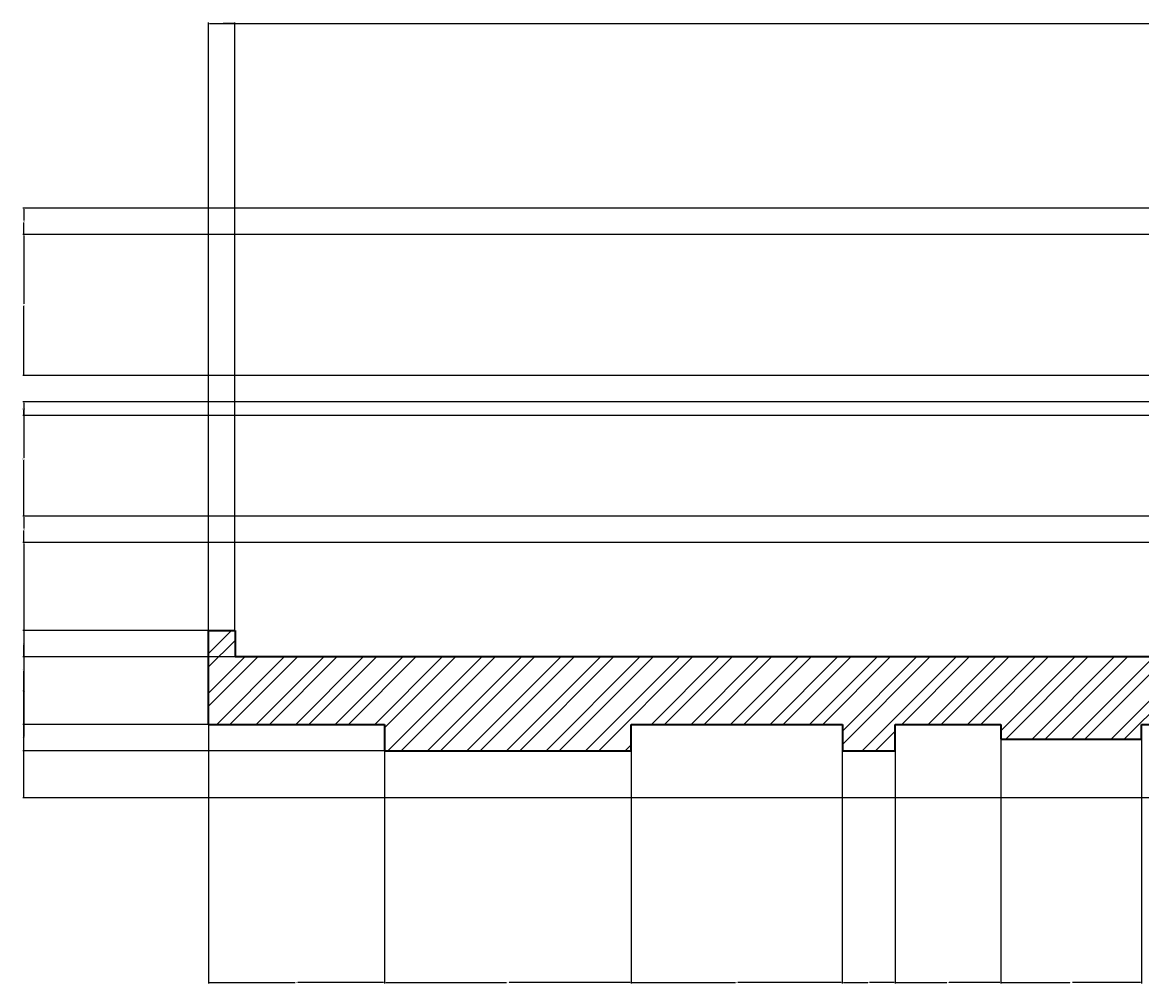
# Model space of a CAD drawing. Units: inches. Extents: x 2121 to 2815, y 1818 to 2233.
# Tile 3 of 6: x 2121 to 2312, y 2070 to 2233. Entities that reach past the tile are written whole.
import ezdxf

# ---------------------------------------------------------------- set-up
doc = ezdxf.new("R2010")
doc.units = ezdxf.units.IN
for name, color, linetype, lineweight in [('A-ANNO-DIMS', 2, 'Continuous', 18), ('A-WALL', 7, 'Continuous', 35), ('A-WALL-PATT', 8, 'Continuous', 13)]:
    doc.layers.add(name, color=color, linetype=linetype, lineweight=lineweight)
doc.styles.get("Standard").update_dxf_attribs({"font": 'arial.ttf'})
doc.dimstyles.get("Standard").update_dxf_attribs({"dimtxt": 0.18, "dimasz": 0.18, "dimexe": 0.18, "dimexo": 0.0625, "dimgap": 0.09, "dimtad": 0, "dimtih": 1, "dimtoh": 1, "dimdec": 4, "dimzin": 0, "dimdsep": 46, "dimtxsty": 'Standard', "dimcen": 0.09, "dimadec": 0, "dimazin": 0, "dimtfac": 1, "dimtdec": 4, "dimtofl": 0, "dimtmove": 0, "dimatfit": 3, "dimfxl": 1, "dimtolj": 1, "dimtzin": 0, "dimarcsym": 0})

# ---------------------------------------------------------------- blocks, each defined once
blk = doc.blocks.new('*D10')
at = {"layer": 'A-ANNO-DIMS', "color": 0, "lineweight": -2, "transparency": 16777216}
for p, q in [((2152.83, 2129.87), (2152.83, 2233.48)), ((2153.01, 2233.3), (2396.54, 2233.3)), ((2640.65, 2233.3), (2397.13, 2233.3)), ((2640.83, 2129.87), (2640.83, 2233.48))]:
    blk.add_line(p, q, dxfattribs=at)
at = {"layer": 'A-ANNO-DIMS', "color": 0, "transparency": 16777216}
for points in [[(2153.01, 2233.33), (2153.01, 2233.27), (2152.83, 2233.3)], [(2640.65, 2233.33), (2640.65, 2233.27), (2640.83, 2233.3)]]:
    blk.add_solid(points, dxfattribs=at)
at = {"layer": 'Defpoints', "color": 0, "transparency": 16777216}
for p in [(2640.83, 2233.3), (2152.83, 2129.81), (2640.83, 2129.81)]:
    blk.add_point(p, dxfattribs=at)
at = {"layer": 'A-ANNO-DIMS', "color": 0, "transparency": 16777216, "insert": (2396.83, 2233.3), "char_height": 0.18, "attachment_point": 5}
blk.add_mtext('\\A1;488', dxfattribs=at)
blk = doc.blocks.new('*D12')
at = {"layer": 'A-ANNO-DIMS', "color": 0, "lineweight": -2, "transparency": 16777216}
for p, q in [((2152.83, 2113.75), (2152.83, 2069.63)), ((2182.83, 2109.25), (2182.83, 2069.63)), ((2153.01, 2069.81), (2167.61, 2069.81)), ((2182.65, 2069.81), (2168.05, 2069.81))]:
    blk.add_line(p, q, dxfattribs=at)
at = {"layer": 'A-ANNO-DIMS', "color": 0, "transparency": 16777216}
for points in [[(2153.01, 2069.84), (2153.01, 2069.78), (2152.83, 2069.81)], [(2182.65, 2069.84), (2182.65, 2069.78), (2182.83, 2069.81)]]:
    blk.add_solid(points, dxfattribs=at)
at = {"layer": 'Defpoints', "color": 0, "transparency": 16777216}
for p in [(2152.83, 2113.81), (2182.83, 2109.31), (2182.83, 2069.81)]:
    blk.add_point(p, dxfattribs=at)
at = {"layer": 'A-ANNO-DIMS', "color": 0, "transparency": 16777216, "insert": (2167.83, 2069.81), "char_height": 0.18, "attachment_point": 5}
blk.add_mtext('\\A1;30', dxfattribs=at)
blk = doc.blocks.new('*D13')
at = {"layer": 'A-ANNO-DIMS', "color": 0, "lineweight": -2, "transparency": 16777216}
for p, q in [((2182.83, 2109.25), (2182.83, 2069.63)), ((2224.83, 2109.25), (2224.83, 2069.63)), ((2183.01, 2069.81), (2203.61, 2069.81)), ((2224.65, 2069.81), (2204.05, 2069.81))]:
    blk.add_line(p, q, dxfattribs=at)
at = {"layer": 'A-ANNO-DIMS', "color": 0, "transparency": 16777216}
for points in [[(2183.01, 2069.84), (2183.01, 2069.78), (2182.83, 2069.81)], [(2224.65, 2069.84), (2224.65, 2069.78), (2224.83, 2069.81)]]:
    blk.add_solid(points, dxfattribs=at)
at = {"layer": 'Defpoints', "color": 0, "transparency": 16777216}
for p in [(2182.83, 2109.31), (2224.83, 2109.31), (2224.83, 2069.81)]:
    blk.add_point(p, dxfattribs=at)
at = {"layer": 'A-ANNO-DIMS', "color": 0, "transparency": 16777216, "insert": (2203.83, 2069.81), "char_height": 0.18, "attachment_point": 5}
blk.add_mtext('\\A1;42', dxfattribs=at)
blk = doc.blocks.new('*D14')
at = {"layer": 'A-ANNO-DIMS', "color": 0, "lineweight": -2, "transparency": 16777216}
for p, q in [((2224.83, 2109.25), (2224.83, 2069.63)), ((2260.83, 2109.25), (2260.83, 2069.63)), ((2225.01, 2069.81), (2242.61, 2069.81)), ((2260.65, 2069.81), (2243.05, 2069.81))]:
    blk.add_line(p, q, dxfattribs=at)
at = {"layer": 'A-ANNO-DIMS', "color": 0, "transparency": 16777216}
for points in [[(2225.01, 2069.84), (2225.01, 2069.78), (2224.83, 2069.81)], [(2260.65, 2069.84), (2260.65, 2069.78), (2260.83, 2069.81)]]:
    blk.add_solid(points, dxfattribs=at)
at = {"layer": 'Defpoints', "color": 0, "transparency": 16777216}
for p in [(2224.83, 2109.31), (2260.83, 2109.31), (2260.83, 2069.81)]:
    blk.add_point(p, dxfattribs=at)
at = {"layer": 'A-ANNO-DIMS', "color": 0, "transparency": 16777216, "insert": (2242.83, 2069.81), "char_height": 0.18, "attachment_point": 5}
blk.add_mtext('\\A1;36', dxfattribs=at)
blk = doc.blocks.new('*D15')
at = {"layer": 'A-ANNO-DIMS', "color": 0, "lineweight": -2, "transparency": 16777216}
for p, q in [((2260.83, 2109.25), (2260.83, 2069.63)), ((2269.83, 2109.25), (2269.83, 2069.63)), ((2261.01, 2069.81), (2265.18, 2069.81)), ((2269.65, 2069.81), (2265.48, 2069.81))]:
    blk.add_line(p, q, dxfattribs=at)
at = {"layer": 'A-ANNO-DIMS', "color": 0, "transparency": 16777216}
for points in [[(2261.01, 2069.84), (2261.01, 2069.78), (2260.83, 2069.81)], [(2269.65, 2069.84), (2269.65, 2069.78), (2269.83, 2069.81)]]:
    blk.add_solid(points, dxfattribs=at)
at = {"layer": 'Defpoints', "color": 0, "transparency": 16777216}
for p in [(2260.83, 2109.31), (2269.83, 2109.31), (2269.83, 2069.81)]:
    blk.add_point(p, dxfattribs=at)
at = {"layer": 'A-ANNO-DIMS', "color": 0, "transparency": 16777216, "insert": (2265.33, 2069.81), "char_height": 0.18, "attachment_point": 5}
blk.add_mtext('\\A1;9', dxfattribs=at)
blk = doc.blocks.new('*D16')
at = {"layer": 'A-ANNO-DIMS', "color": 0, "lineweight": -2, "transparency": 16777216}
for p, q in [((2287.83, 2111.25), (2287.83, 2069.63)), ((2269.83, 2109.25), (2269.83, 2069.63)), ((2270.01, 2069.81), (2278.62, 2069.81)), ((2287.65, 2069.81), (2279.04, 2069.81))]:
    blk.add_line(p, q, dxfattribs=at)
at = {"layer": 'A-ANNO-DIMS', "color": 0, "transparency": 16777216}
for points in [[(2270.01, 2069.84), (2270.01, 2069.78), (2269.83, 2069.81)], [(2287.65, 2069.84), (2287.65, 2069.78), (2287.83, 2069.81)]]:
    blk.add_solid(points, dxfattribs=at)
at = {"layer": 'Defpoints', "color": 0, "transparency": 16777216}
for p in [(2287.83, 2111.31), (2269.83, 2109.31), (2287.83, 2069.81)]:
    blk.add_point(p, dxfattribs=at)
at = {"layer": 'A-ANNO-DIMS', "color": 0, "transparency": 16777216, "insert": (2278.83, 2069.81), "char_height": 0.18, "attachment_point": 5}
blk.add_mtext('\\A1;18', dxfattribs=at)
blk = doc.blocks.new('*D17')
at = {"layer": 'A-ANNO-DIMS', "color": 0, "lineweight": -2, "transparency": 16777216}
for p, q in [((2287.83, 2111.25), (2287.83, 2069.63)), ((2311.83, 2111.25), (2311.83, 2069.63)), ((2288.01, 2069.81), (2299.61, 2069.81)), ((2311.65, 2069.81), (2300.05, 2069.81))]:
    blk.add_line(p, q, dxfattribs=at)
at = {"layer": 'A-ANNO-DIMS', "color": 0, "transparency": 16777216}
for points in [[(2288.01, 2069.84), (2288.01, 2069.78), (2287.83, 2069.81)], [(2311.65, 2069.84), (2311.65, 2069.78), (2311.83, 2069.81)]]:
    blk.add_solid(points, dxfattribs=at)
at = {"layer": 'Defpoints', "color": 0, "transparency": 16777216}
for p in [(2287.83, 2111.31), (2311.83, 2111.31), (2311.83, 2069.81)]:
    blk.add_point(p, dxfattribs=at)
at = {"layer": 'A-ANNO-DIMS', "color": 0, "transparency": 16777216, "insert": (2299.83, 2069.81), "char_height": 0.18, "attachment_point": 5}
blk.add_mtext('\\A1;24', dxfattribs=at)
blk = doc.blocks.new('*D28')
at = {"layer": 'A-ANNO-DIMS', "color": 0, "lineweight": -2, "transparency": 16777216}
for p, q in [((2152.83, 2129.87), (2152.83, 2233.48)), ((2153.01, 2233.3), (2154.82, 2233.3)), ((2157.15, 2233.3), (2155.34, 2233.3)), ((2157.33, 2129.87), (2157.33, 2233.48))]:
    blk.add_line(p, q, dxfattribs=at)
at = {"layer": 'A-ANNO-DIMS', "color": 0, "transparency": 16777216}
for points in [[(2153.01, 2233.33), (2153.01, 2233.27), (2152.83, 2233.3)], [(2157.15, 2233.33), (2157.15, 2233.27), (2157.33, 2233.3)]]:
    blk.add_solid(points, dxfattribs=at)
at = {"layer": 'Defpoints', "color": 0, "transparency": 16777216}
for p in [(2157.33, 2233.3), (2152.83, 2129.81), (2157.33, 2129.81)]:
    blk.add_point(p, dxfattribs=at)
at = {"layer": 'A-ANNO-DIMS', "color": 0, "transparency": 16777216, "insert": (2155.08, 2233.3), "char_height": 0.18, "attachment_point": 5}
blk.add_mtext('\\A1;4.5', dxfattribs=at)
blk = doc.blocks.new('*D29')
at = {"layer": 'A-ANNO-DIMS', "color": 0, "lineweight": -2, "transparency": 16777216}
for p, q in [((2157.27, 2129.81), (2121.16, 2129.81)), ((2121.34, 2129.63), (2121.34, 2127.74)), ((2121.34, 2125.49), (2121.34, 2127.38)), ((2157.27, 2125.31), (2121.16, 2125.31))]:
    blk.add_line(p, q, dxfattribs=at)
at = {"layer": 'A-ANNO-DIMS', "color": 0, "transparency": 16777216}
for points in [[(2121.31, 2129.63), (2121.37, 2129.63), (2121.34, 2129.81)], [(2121.31, 2125.49), (2121.37, 2125.49), (2121.34, 2125.31)]]:
    blk.add_solid(points, dxfattribs=at)
at = {"layer": 'Defpoints', "color": 0, "transparency": 16777216}
for p in [(2121.34, 2129.81), (2157.33, 2129.81), (2157.33, 2125.31)]:
    blk.add_point(p, dxfattribs=at)
at = {"layer": 'A-ANNO-DIMS', "color": 0, "transparency": 16777216, "insert": (2121.34, 2127.56), "char_height": 0.18, "attachment_point": 5}
blk.add_mtext('\\A1;4.5', dxfattribs=at)
blk = doc.blocks.new('*D30')
at = {"layer": 'A-ANNO-DIMS', "color": 0, "lineweight": -2, "transparency": 16777216}
for p, q in [((2157.27, 2125.31), (2121.16, 2125.31)), ((2121.34, 2125.13), (2121.34, 2119.74)), ((2121.34, 2113.99), (2121.34, 2119.38)), ((2152.77, 2113.81), (2121.16, 2113.81))]:
    blk.add_line(p, q, dxfattribs=at)
at = {"layer": 'A-ANNO-DIMS', "color": 0, "transparency": 16777216}
for points in [[(2121.31, 2125.13), (2121.37, 2125.13), (2121.34, 2125.31)], [(2121.31, 2113.99), (2121.37, 2113.99), (2121.34, 2113.81)]]:
    blk.add_solid(points, dxfattribs=at)
at = {"layer": 'Defpoints', "color": 0, "transparency": 16777216}
for p in [(2157.33, 2125.31), (2121.34, 2113.81), (2152.83, 2113.81)]:
    blk.add_point(p, dxfattribs=at)
at = {"layer": 'A-ANNO-DIMS', "color": 0, "transparency": 16777216, "insert": (2121.34, 2119.56), "char_height": 0.18, "attachment_point": 5}
blk.add_mtext('\\A1;11.5', dxfattribs=at)
blk = doc.blocks.new('*D31')
at = {"layer": 'A-ANNO-DIMS', "color": 0, "lineweight": -2, "transparency": 16777216}
for p, q in [((2182.77, 2113.81), (2121.16, 2113.81)), ((2121.34, 2113.63), (2121.34, 2111.74)), ((2121.34, 2109.49), (2121.34, 2111.38)), ((2182.77, 2109.31), (2121.16, 2109.31))]:
    blk.add_line(p, q, dxfattribs=at)
at = {"layer": 'A-ANNO-DIMS', "color": 0, "transparency": 16777216}
for points in [[(2121.31, 2113.63), (2121.37, 2113.63), (2121.34, 2113.81)], [(2121.31, 2109.49), (2121.37, 2109.49), (2121.34, 2109.31)]]:
    blk.add_solid(points, dxfattribs=at)
at = {"layer": 'Defpoints', "color": 0, "transparency": 16777216}
for p in [(2182.83, 2113.81), (2121.34, 2109.31), (2182.83, 2109.31)]:
    blk.add_point(p, dxfattribs=at)
at = {"layer": 'A-ANNO-DIMS', "color": 0, "transparency": 16777216, "insert": (2121.34, 2111.56), "char_height": 0.18, "attachment_point": 5}
blk.add_mtext('\\A1;4.5', dxfattribs=at)
blk = doc.blocks.new('*D36')
at = {"layer": 'A-ANNO-DIMS', "color": 0, "lineweight": -2, "transparency": 16777216}
for p, q in [((2515.77, 2125.31), (2121.16, 2125.31)), ((2121.34, 2125.13), (2121.34, 2113.49)), ((2121.34, 2101.49), (2121.34, 2113.13)), ((2491.77, 2101.31), (2121.16, 2101.31))]:
    blk.add_line(p, q, dxfattribs=at)
at = {"layer": 'A-ANNO-DIMS', "color": 0, "transparency": 16777216}
for points in [[(2121.31, 2125.13), (2121.37, 2125.13), (2121.34, 2125.31)], [(2121.31, 2101.49), (2121.37, 2101.49), (2121.34, 2101.31)]]:
    blk.add_solid(points, dxfattribs=at)
at = {"layer": 'Defpoints', "color": 0, "transparency": 16777216}
for p in [(2121.34, 2125.31), (2515.83, 2125.31), (2491.83, 2101.31)]:
    blk.add_point(p, dxfattribs=at)
at = {"layer": 'A-ANNO-DIMS', "color": 0, "transparency": 16777216, "insert": (2121.34, 2113.31), "char_height": 0.18, "attachment_point": 5}
blk.add_mtext('\\A1;24', dxfattribs=at)
blk = doc.blocks.new('*D86')
at = {"layer": 'A-ANNO-DIMS', "color": 0, "lineweight": -2, "transparency": 16777216}
for p, q in [((2760.77, 2144.81), (2121.16, 2144.81)), ((2121.34, 2144.63), (2121.34, 2123.24)), ((2121.34, 2101.49), (2121.34, 2122.88)), ((2760.77, 2101.31), (2121.16, 2101.31))]:
    blk.add_line(p, q, dxfattribs=at)
at = {"layer": 'A-ANNO-DIMS', "color": 0, "transparency": 16777216}
for points in [[(2121.31, 2144.63), (2121.37, 2144.63), (2121.34, 2144.81)], [(2121.31, 2101.49), (2121.37, 2101.49), (2121.34, 2101.31)]]:
    blk.add_solid(points, dxfattribs=at)
at = {"layer": 'Defpoints', "color": 0, "transparency": 16777216}
for p in [(2121.34, 2144.81), (2760.83, 2144.81), (2760.83, 2101.31)]:
    blk.add_point(p, dxfattribs=at)
at = {"layer": 'A-ANNO-DIMS', "color": 0, "transparency": 16777216, "insert": (2121.34, 2123.06), "char_height": 0.18, "attachment_point": 5}
blk.add_mtext('\\A1;43.5', dxfattribs=at)
blk = doc.blocks.new('*D88')
at = {"layer": 'A-ANNO-DIMS', "color": 0, "lineweight": -2, "transparency": 16777216}
for p, q in [((2760.77, 2197.31), (2121.16, 2197.31)), ((2121.34, 2197.13), (2121.34, 2185.49)), ((2121.34, 2173.49), (2121.34, 2185.13)), ((2760.77, 2173.31), (2121.16, 2173.31))]:
    blk.add_line(p, q, dxfattribs=at)
at = {"layer": 'A-ANNO-DIMS', "color": 0, "transparency": 16777216}
for points in [[(2121.31, 2197.13), (2121.37, 2197.13), (2121.34, 2197.31)], [(2121.31, 2173.49), (2121.37, 2173.49), (2121.34, 2173.31)]]:
    blk.add_solid(points, dxfattribs=at)
at = {"layer": 'Defpoints', "color": 0, "transparency": 16777216}
for p in [(2121.34, 2197.31), (2760.83, 2197.31), (2760.83, 2173.31)]:
    blk.add_point(p, dxfattribs=at)
at = {"layer": 'A-ANNO-DIMS', "color": 0, "transparency": 16777216, "insert": (2121.34, 2185.31), "char_height": 0.18, "attachment_point": 5}
blk.add_mtext('\\A1;24', dxfattribs=at)
blk = doc.blocks.new('*D89')
at = {"layer": 'A-ANNO-DIMS', "color": 0, "lineweight": -2, "transparency": 16777216}
for p, q in [((2756.07, 2201.81), (2121.16, 2201.81)), ((2121.34, 2201.63), (2121.34, 2199.74)), ((2121.34, 2197.49), (2121.34, 2199.38)), ((2760.77, 2197.31), (2121.16, 2197.31))]:
    blk.add_line(p, q, dxfattribs=at)
at = {"layer": 'A-ANNO-DIMS', "color": 0, "transparency": 16777216}
for points in [[(2121.31, 2201.63), (2121.37, 2201.63), (2121.34, 2201.81)], [(2121.31, 2197.49), (2121.37, 2197.49), (2121.34, 2197.31)]]:
    blk.add_solid(points, dxfattribs=at)
at = {"layer": 'Defpoints', "color": 0, "transparency": 16777216}
for p in [(2121.34, 2201.81), (2756.14, 2201.81), (2760.83, 2197.31)]:
    blk.add_point(p, dxfattribs=at)
at = {"layer": 'A-ANNO-DIMS', "color": 0, "transparency": 16777216, "insert": (2121.34, 2199.56), "char_height": 0.18, "attachment_point": 5}
blk.add_mtext('\\A1;4.5', dxfattribs=at)
blk = doc.blocks.new('*D90')
at = {"layer": 'A-ANNO-DIMS', "color": 0, "lineweight": -2, "transparency": 16777216}
for p, q in [((2760.77, 2168.81), (2121.16, 2168.81)), ((2121.34, 2168.63), (2121.34, 2159.24)), ((2121.34, 2149.49), (2121.34, 2158.88)), ((2760.77, 2149.31), (2121.16, 2149.31))]:
    blk.add_line(p, q, dxfattribs=at)
at = {"layer": 'A-ANNO-DIMS', "color": 0, "transparency": 16777216}
for points in [[(2121.31, 2168.63), (2121.37, 2168.63), (2121.34, 2168.81)], [(2121.31, 2149.49), (2121.37, 2149.49), (2121.34, 2149.31)]]:
    blk.add_solid(points, dxfattribs=at)
at = {"layer": 'Defpoints', "color": 0, "transparency": 16777216}
for p in [(2121.34, 2168.81), (2760.83, 2168.81), (2760.83, 2149.31)]:
    blk.add_point(p, dxfattribs=at)
at = {"layer": 'A-ANNO-DIMS', "color": 0, "transparency": 16777216, "insert": (2121.34, 2159.06), "char_height": 0.18, "attachment_point": 5}
blk.add_mtext('\\A1;19.5', dxfattribs=at)
blk = doc.blocks.new('*D91')
at = {"layer": 'A-ANNO-DIMS', "color": 0, "lineweight": -2, "transparency": 16777216}
for p, q in [((2760.77, 2149.31), (2121.16, 2149.31)), ((2121.34, 2149.13), (2121.34, 2147.24)), ((2121.34, 2144.99), (2121.34, 2146.88)), ((2760.77, 2144.81), (2121.16, 2144.81))]:
    blk.add_line(p, q, dxfattribs=at)
at = {"layer": 'A-ANNO-DIMS', "color": 0, "transparency": 16777216}
for points in [[(2121.31, 2149.13), (2121.37, 2149.13), (2121.34, 2149.31)], [(2121.31, 2144.99), (2121.37, 2144.99), (2121.34, 2144.81)]]:
    blk.add_solid(points, dxfattribs=at)
at = {"layer": 'Defpoints', "color": 0, "transparency": 16777216}
for p in [(2121.34, 2149.31), (2760.83, 2149.31), (2760.83, 2144.81)]:
    blk.add_point(p, dxfattribs=at)
at = {"layer": 'A-ANNO-DIMS', "color": 0, "transparency": 16777216, "insert": (2121.34, 2147.06), "char_height": 0.18, "attachment_point": 5}
blk.add_mtext('\\A1;4.5', dxfattribs=at)
blk = doc.blocks.new('*D97')
at = {"layer": 'A-ANNO-DIMS', "color": 0, "lineweight": -2, "transparency": 16777216}
for p, q in [((2765.42, 2168.81), (2121.16, 2168.81)), ((2121.34, 2168.63), (2121.34, 2167.83)), ((2121.34, 2166.66), (2121.34, 2167.46)), ((2765.42, 2166.48), (2121.16, 2166.48))]:
    blk.add_line(p, q, dxfattribs=at)
at = {"layer": 'A-ANNO-DIMS', "color": 0, "transparency": 16777216}
for points in [[(2121.31, 2168.63), (2121.37, 2168.63), (2121.34, 2168.81)], [(2121.31, 2166.66), (2121.37, 2166.66), (2121.34, 2166.48)]]:
    blk.add_solid(points, dxfattribs=at)
at = {"layer": 'Defpoints', "color": 0, "transparency": 16777216}
for p in [(2121.34, 2168.81), (2765.49, 2168.81), (2765.49, 2166.48)]:
    blk.add_point(p, dxfattribs=at)
at = {"layer": 'A-ANNO-DIMS', "color": 0, "transparency": 16777216, "insert": (2121.34, 2167.64), "char_height": 0.18, "attachment_point": 5}
blk.add_mtext('\\A1;2.33', dxfattribs=at)

msp = doc.modelspace()

# ---------------------------------------------------------------- hatches: boundary and pattern name
at = {"layer": 'A-WALL-PATT'}
h = msp.add_hatch(dxfattribs=at)
h.set_pattern_fill('ANSI32', color=256, scale=0.5)
h.paths.add_polyline_path([(2496.3326, 2122.9949), (2511.3326, 2122.9949), (2511.3326, 2117.8278), (2515.8326, 2122.3278), (2515.8326, 2125.309), (2157.3326, 2125.309), (2157.3326, 2129.809), (2152.8326, 2129.809), (2152.8326, 2125.309), (2152.8326, 2113.809), (2182.8326, 2113.809), (2182.8326, 2109.309), (2224.8326, 2109.309), (2224.8326, 2113.809), (2260.8326, 2113.809), (2260.8326, 2109.309), (2269.8326, 2109.309), (2269.8326, 2113.809), (2287.8326, 2113.809), (2287.8326, 2111.309), (2311.8326, 2111.309), (2311.8326, 2113.809), (2344.8326, 2113.809), (2344.8326, 2118.309), (2386.8326, 2118.309), (2386.8326, 2113.809), (2401.8326, 2113.809), (2401.8326, 2109.309), (2419.8326, 2109.309), (2419.8326, 2118.309), (2437.8326, 2118.309), (2437.8326, 2113.809), (2461.8326, 2113.809), (2461.8326, 2116.309), (2491.8326, 2116.309), (2491.8326, 2101.309), (2494.8138, 2101.309), (2496.3326, 2102.8278)])
h.paths.add_polyline_path([(2640.8326, 2129.809), (2628.8326, 2129.809), (2628.8326, 2125.309), (2619.8326, 2125.309), (2619.8326, 2108.3582), (2628.8326, 2101.309), (2640.8326, 2101.309)])

# ---------------------------------------------------------------- linework, layer by layer
at = {"layer": 'A-WALL'}
for p, q in [((2152.8326, 2125.309), (2152.8326, 2129.809)), ((2152.8326, 2129.809), (2157.3326, 2129.809)), ((2157.3326, 2129.809), (2157.3326, 2125.309)), ((2152.8326, 2113.809), (2152.8326, 2125.309)), ((2515.8326, 2125.309), (2157.3326, 2125.309)), ((2152.8326, 2113.809), (2182.8326, 2113.809)), ((2182.8326, 2113.809), (2182.8326, 2109.309)), ((2224.8326, 2109.309), (2224.8326, 2113.809)), ((2224.8326, 2113.809), (2260.8326, 2113.809)), ((2260.8326, 2113.809), (2260.8326, 2109.309)), ((2269.8326, 2109.309), (2269.8326, 2113.809)), ((2269.8326, 2113.809), (2287.8326, 2113.809)), ((2287.8326, 2113.809), (2287.8326, 2111.309)), ((2311.8326, 2111.309), (2311.8326, 2113.809)), ((2311.8326, 2113.809), (2344.8326, 2113.809)), ((2287.8326, 2111.309), (2311.8326, 2111.309)), ((2182.8326, 2109.309), (2224.8326, 2109.309)), ((2260.8326, 2109.309), (2269.8326, 2109.309))]:
    msp.add_line(p, q, dxfattribs=at)

# ---------------------------------------------------------------- dimensions: what is measured, and where the dimension line sits
at = {"layer": 'A-ANNO-DIMS'}
for base, p1, p2, override, picture, middle in [((2640.8326, 2233.304), (2152.8326, 2129.809), (2640.8326, 2129.809), {"dimdec": 0, "dimlfac": 1, "dimrnd": 0, "dimzin": 0, "dimdsep": 46, "dimlunit": 2}, '*D10', (2396.8326, 2233.304)), ((2157.3326, 2233.304), (2152.8326, 2129.809), (2157.3326, 2129.809), {"dimdec": 1, "dimlfac": 1, "dimrnd": 0, "dimzin": 0, "dimdsep": 46, "dimlunit": 2}, '*D28', (2155.0826, 2233.304)), ((2182.8326, 2069.814), (2152.8326, 2113.809), (2182.8326, 2109.309), {"dimdec": 0, "dimlfac": 1, "dimrnd": 0, "dimzin": 0, "dimdsep": 46, "dimlunit": 2}, '*D12', (2167.8326, 2069.814)), ((2287.8326, 2069.814), (2269.8326, 2109.309), (2287.8326, 2111.309), {"dimdec": 0, "dimlfac": 1, "dimrnd": 0, "dimzin": 0, "dimdsep": 46, "dimlunit": 2}, '*D16', (2278.8326, 2069.814)), ((2311.8326, 2069.814), (2287.8326, 2111.309), (2311.8326, 2111.309), {"dimdec": 0, "dimlfac": 1, "dimrnd": 0, "dimzin": 0, "dimdsep": 46, "dimlunit": 2}, '*D17', (2299.8326, 2069.814)), ((2224.8326, 2069.814), (2182.8326, 2109.309), (2224.8326, 2109.309), {"dimdec": 0, "dimlfac": 1, "dimrnd": 0, "dimzin": 0, "dimdsep": 46, "dimlunit": 2}, '*D13', (2203.8326, 2069.814)), ((2260.8326, 2069.814), (2224.8326, 2109.309), (2260.8326, 2109.309), {"dimdec": 0, "dimlfac": 1, "dimrnd": 0, "dimzin": 0, "dimdsep": 46, "dimlunit": 2}, '*D14', (2242.8326, 2069.814)), ((2269.8326, 2069.814), (2260.8326, 2109.309), (2269.8326, 2109.309), {"dimdec": 0, "dimlfac": 1, "dimrnd": 0, "dimzin": 0, "dimdsep": 46, "dimlunit": 2}, '*D15', (2265.3326, 2069.814))]:
    dim = msp.add_linear_dim(base=base, p1=p1, p2=p2, dimstyle='Standard', override=override, dxfattribs=at)
    dim.commit()
    dim.dimension.update_dxf_attribs({"geometry": picture, "text_midpoint": middle})
for base, p1, p2, override, picture, middle in [((2121.3376, 2201.809), (2760.8326, 2197.309), (2756.1373, 2201.809), {"dimdec": 1, "dimlfac": 1, "dimrnd": 0, "dimzin": 0, "dimdsep": 46, "dimlunit": 2}, '*D89', (2121.3376, 2199.559)), ((2121.3376, 2197.309), (2760.8326, 2173.309), (2760.8326, 2197.309), {"dimdec": 0, "dimlfac": 1, "dimrnd": 0, "dimzin": 0, "dimdsep": 46, "dimlunit": 2}, '*D88', (2121.3376, 2185.309)), ((2121.3376, 2168.809), (2760.8326, 2149.309), (2760.8326, 2168.809), {"dimdec": 1, "dimlfac": 1, "dimrnd": 0, "dimzin": 0, "dimdsep": 46, "dimlunit": 2}, '*D90', (2121.3376, 2159.059)), ((2121.3376, 2168.809), (2765.4865, 2166.4788), (2765.4865, 2168.809), {"dimdec": 2, "dimlfac": 1, "dimrnd": 0, "dimzin": 0, "dimdsep": 46, "dimlunit": 2}, '*D97', (2121.3376, 2167.6439)), ((2121.3376, 2149.309), (2760.8326, 2144.809), (2760.8326, 2149.309), {"dimdec": 1, "dimlfac": 1, "dimrnd": 0, "dimzin": 0, "dimdsep": 46, "dimlunit": 2}, '*D91', (2121.3376, 2147.059)), ((2121.3376, 2144.809), (2760.8326, 2101.309), (2760.8326, 2144.809), {"dimdec": 1, "dimlfac": 1, "dimrnd": 0, "dimzin": 0, "dimdsep": 46, "dimlunit": 2}, '*D86', (2121.3376, 2123.059)), ((2121.3376, 2129.809), (2157.3326, 2125.309), (2157.3326, 2129.809), {"dimdec": 1, "dimlfac": 1, "dimrnd": 0, "dimzin": 0, "dimdsep": 46, "dimlunit": 2}, '*D29', (2121.3376, 2127.559)), ((2121.3376, 2113.809), (2157.3326, 2125.309), (2152.8326, 2113.809), {"dimdec": 1, "dimlfac": 1, "dimrnd": 0, "dimzin": 0, "dimdsep": 46, "dimlunit": 2}, '*D30', (2121.3376, 2119.559)), ((2121.3376, 2125.309), (2491.8326, 2101.309), (2515.8326, 2125.309), {"dimdec": 0, "dimlfac": 1, "dimrnd": 0, "dimzin": 0, "dimdsep": 46, "dimlunit": 2}, '*D36', (2121.3376, 2113.309)), ((2121.3376, 2109.309), (2182.8326, 2113.809), (2182.8326, 2109.309), {"dimdec": 1, "dimlfac": 1, "dimrnd": 0, "dimzin": 0, "dimdsep": 46, "dimlunit": 2}, '*D31', (2121.3376, 2111.559))]:
    dim = msp.add_linear_dim(base=base, p1=p1, p2=p2, angle=90, dimstyle='Standard', override=override, dxfattribs=at)
    dim.commit()
    dim.dimension.update_dxf_attribs({"geometry": picture, "text_midpoint": middle})

doc.saveas('drawing.dxf')
